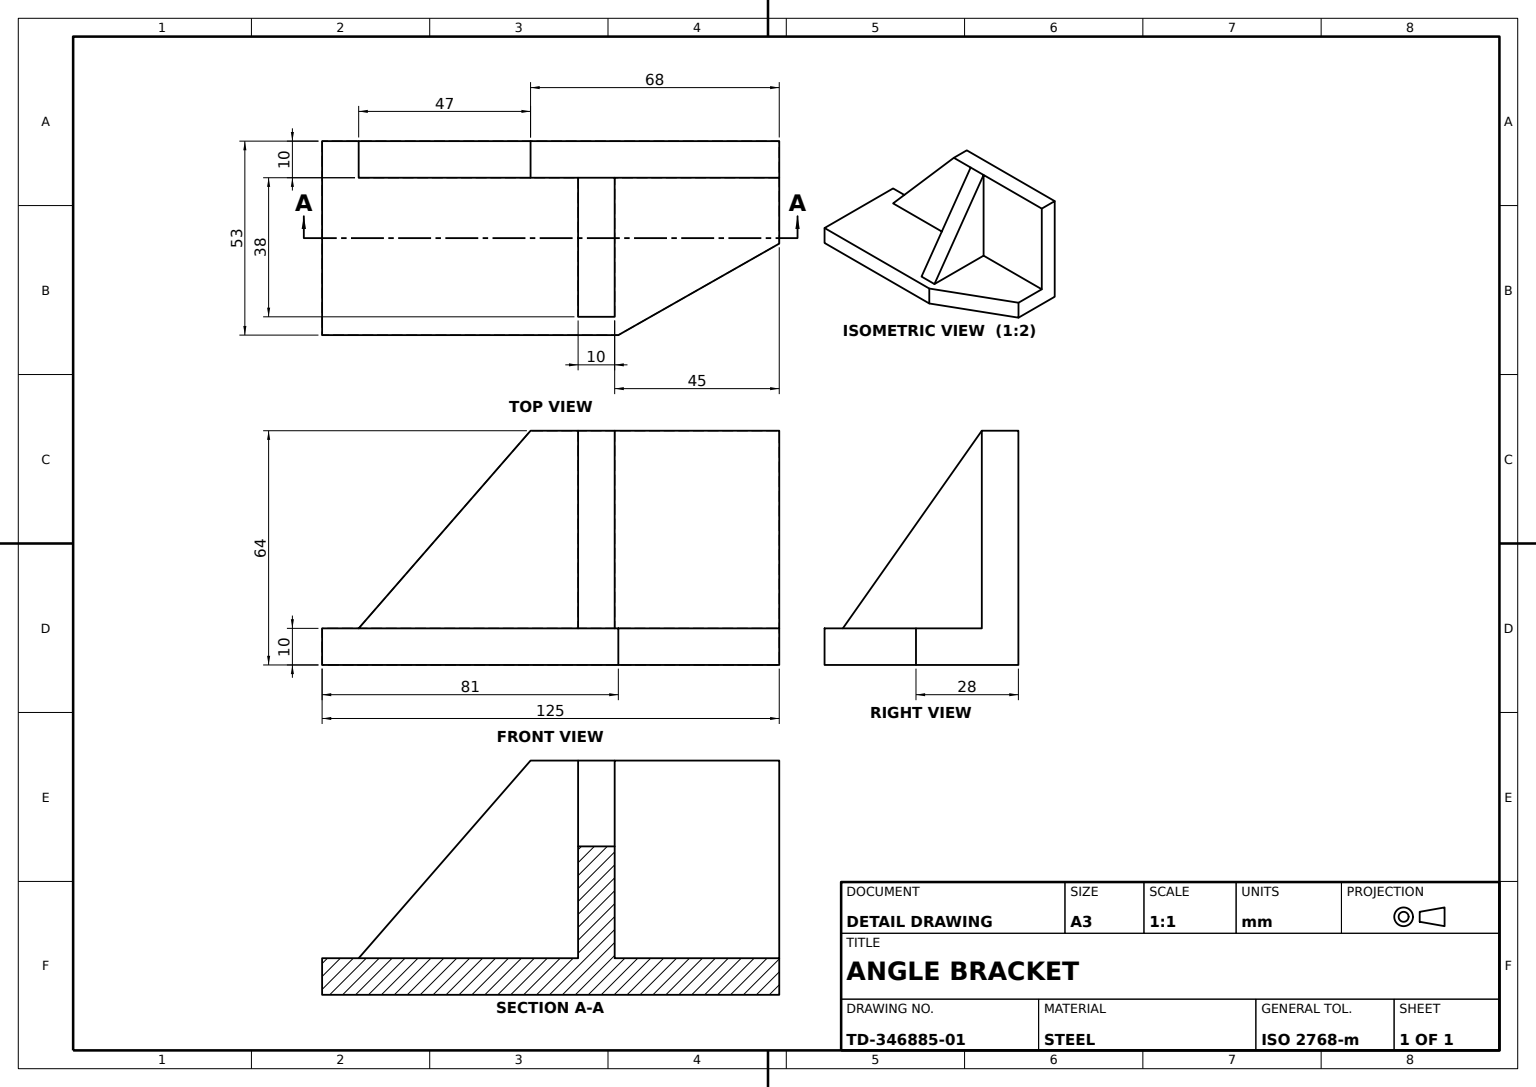
from build123d import *

# Parameters (mm, degrees)
BASE_PLATE_DEPTH       = 5
RAISED_PAD_DEPTH       = 10
UPRIGHT_WALL_PROFILE_W = 10
UPRIGHT_WALL_PROFILE_H = 38
UPRIGHT_WALL_DEPTH     = 54
GUSSET_CUT_DEPTH       = 10


with BuildPart() as part:
    # Base Plate Profile → Base Plate (new, symmetric)
    with BuildSketch(Plane(origin=(0, 0, 0), x_dir=(1, 0, 0), z_dir=(0, 1, 0))):
        Polygon((0, 0), (81, 0), (125, 25), (125, 53), (0, 53), align=None)
    extrude(amount=BASE_PLATE_DEPTH, both=True)

    # Raised Pad Profile → Raised Pad (add)
    with BuildSketch(Plane(origin=(0, 0, -53), x_dir=(-1, 0, 0), z_dir=(0, 0, -1))):
        Polygon((-125, 5), (-10, 5), (-57, 59), (-125, 59), align=None)
    extrude(amount=-RAISED_PAD_DEPTH)

    # Upright Wall Profile → Upright Wall (add)
    with BuildSketch(Plane(origin=(0, 5, 0), x_dir=(1, 0, 0), z_dir=(0, 1, 0))):
        with Locations((75, 24)):
            Rectangle(UPRIGHT_WALL_PROFILE_W, UPRIGHT_WALL_PROFILE_H)
    extrude(amount=UPRIGHT_WALL_DEPTH)

    # Gusset Cut Profile → Gusset Cut (cut)
    with BuildSketch(Plane(origin=(80, 0, 0), x_dir=(0, 0, -1), z_dir=(1, 0, 0))):
        Polygon((43, 59), (5, 5), (5, 59), align=None)
    extrude(amount=-GUSSET_CUT_DEPTH, mode=Mode.SUBTRACT)


solid = part.part
